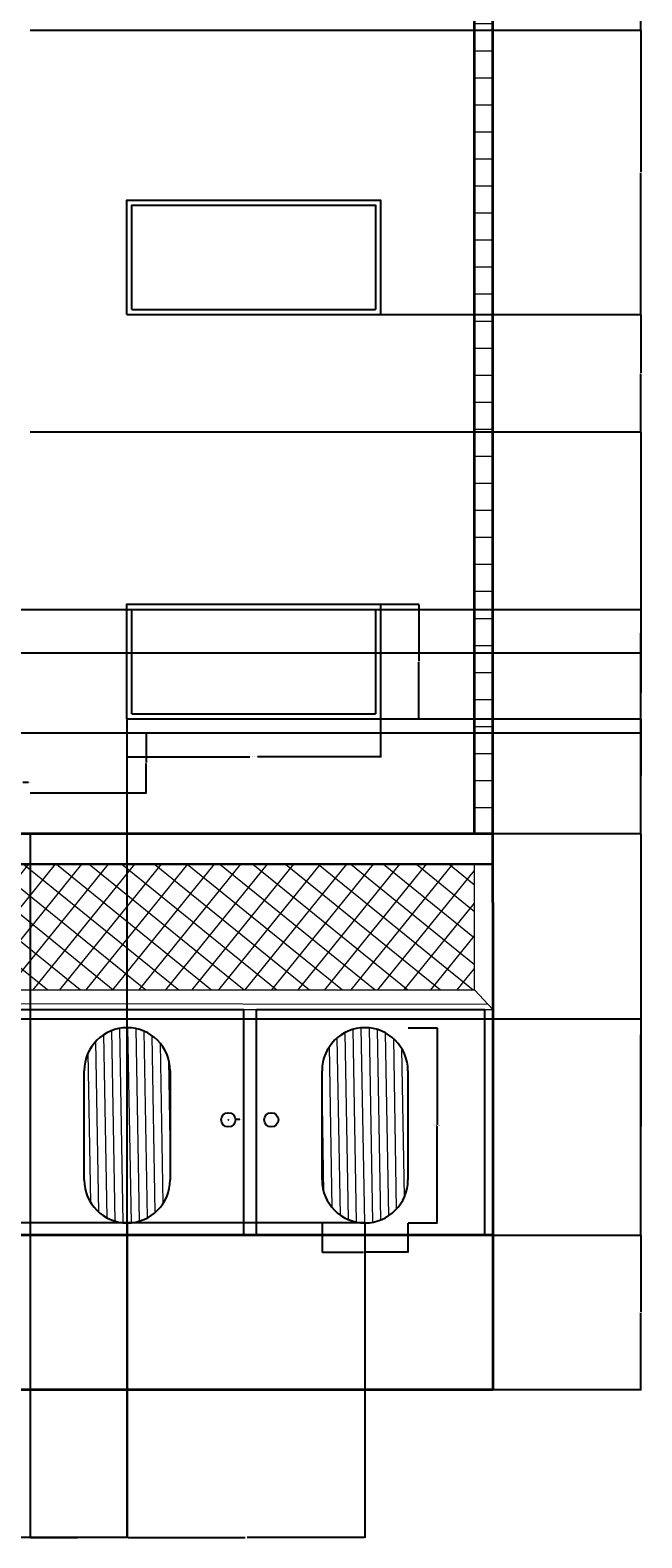
# Model space of a CAD drawing. Units: inches. Extents: x 373 to 969, y 157 to 1341.
# Tile 2 of 3: x 731 to 969, y 157 to 743. Entities that reach past the tile are written whole.
import ezdxf

# ---------------------------------------------------------------- set-up
doc = ezdxf.new("R2010")
doc.units = ezdxf.units.IN
doc.header["$MEASUREMENT"] = 0
for name, color, linetype, lineweight in [('A-ANNO-DIMS', 2, 'Continuous', 18), ('A-DOOR', 3, 'Continuous', 25), ('A-DOOR-PATT', 8, 'Continuous', 13), ('A-ELEV-TRIM', 9, 'Continuous', 18), ('A-FLOR', 7, 'Continuous', 30), ('A-GLAZ', 4, 'Continuous', 25), ('A-WALL', 7, 'Continuous', 35), ('A-WALL-PATT', 8, 'Continuous', 13)]:
    doc.layers.add(name, color=color, linetype=linetype, lineweight=lineweight)
doc.styles.get("Standard").update_dxf_attribs({"font": 'arial.ttf'})
doc.dimstyles.get("Standard").update_dxf_attribs({"dimtxt": 0.18, "dimasz": 0.18, "dimexe": 0.18, "dimexo": 0.0625, "dimgap": 0.09, "dimtad": 0, "dimtih": 1, "dimtoh": 1, "dimdec": 4, "dimzin": 0, "dimdsep": 46, "dimlunit": 4, "dimtxsty": 'Standard', "dimcen": 0.09, "dimadec": 0, "dimazin": 0, "dimtfac": 1, "dimtdec": 4, "dimtofl": 0, "dimtmove": 0, "dimatfit": 3, "dimfxl": 1, "dimtolj": 1, "dimtzin": 0, "dimarcsym": 0})

# ---------------------------------------------------------------- blocks, each defined once
blk = doc.blocks.new('WIN-FIXED-FRAME-ELEV')
for p, q in [((0, 0), (98.59, 0)), ((2, 2), (96.59, 2))]:
    blk.add_line(p, q)
for points in [[(0, 0), (0, 44.5), (98.59, 44.5), (98.59, 0)], [(2, 2), (2, 42.5), (96.59, 42.5), (96.59, 2)]]:
    blk.add_lwpolyline(points)
blk = doc.blocks.new('DOOR-OBROUND-INSERT-ELEV')
for points in [[(0, 16.68), (0, 59.13)], [(33.36, 59.13), (33.36, 16.68)]]:
    blk.add_lwpolyline(points)
for centre, start, end in [((16.68, 59.13), 0, 180), ((16.68, 16.68), 180, 0)]:
    blk.add_arc(centre, 16.68, start, end)
blk = doc.blocks.new('*D7')
at = {"layer": 'A-ANNO-DIMS', "color": 0, "lineweight": -2, "transparency": 16777216}
for p, q in [((768.48, 475.42), (768.48, 460.52)), ((867.07, 475.42), (867.07, 460.52)), ((768.66, 460.7), (816.26, 460.7)), ((866.89, 460.7), (819.29, 460.7))]:
    blk.add_line(p, q, dxfattribs=at)
at = {"layer": 'A-ANNO-DIMS', "color": 0, "transparency": 16777216}
for points in [[(768.66, 460.73), (768.66, 460.67), (768.48, 460.7)], [(866.89, 460.73), (866.89, 460.67), (867.07, 460.7)]]:
    blk.add_solid(points, dxfattribs=at)
at = {"layer": 'Defpoints', "color": 0, "transparency": 16777216}
for p in [(768.48, 475.48), (867.07, 475.48), (867.07, 460.7)]:
    blk.add_point(p, dxfattribs=at)
at = {"layer": 'A-ANNO-DIMS', "color": 0, "transparency": 16777216, "insert": (817.77, 460.7), "char_height": 0.18, "attachment_point": 5}
blk.add_mtext('\\A1;FIXED WINDOW 99 TYP.', dxfattribs=at)
blk = doc.blocks.new('*D8')
at = {"layer": 'A-ANNO-DIMS', "color": 0, "lineweight": -2, "transparency": 16777216}
for p, q in [((867.13, 519.98), (882.04, 519.98)), ((881.86, 519.8), (881.86, 497.92)), ((881.86, 475.66), (881.86, 497.55)), ((867.13, 475.48), (882.04, 475.48))]:
    blk.add_line(p, q, dxfattribs=at)
at = {"layer": 'A-ANNO-DIMS', "color": 0, "transparency": 16777216}
for points in [[(881.83, 519.8), (881.89, 519.8), (881.86, 519.98)], [(881.83, 475.66), (881.89, 475.66), (881.86, 475.48)]]:
    blk.add_solid(points, dxfattribs=at)
at = {"layer": 'Defpoints', "color": 0, "transparency": 16777216}
for p in [(867.07, 519.98), (881.86, 519.98), (867.07, 475.48)]:
    blk.add_point(p, dxfattribs=at)
at = {"layer": 'A-ANNO-DIMS', "color": 0, "transparency": 16777216, "insert": (881.86, 497.73), "char_height": 0.18, "attachment_point": 5}
blk.add_mtext('\\A1;45 TYP.', dxfattribs=at)
blk = doc.blocks.new('*D12')
at = {"layer": 'A-ANNO-DIMS', "color": 0, "lineweight": -2, "transparency": 16777216}
for p, q in [((731, 469.98), (776.15, 469.98)), ((775.97, 469.8), (775.97, 458.53)), ((775.97, 446.9), (775.97, 458.17)), ((731, 446.72), (776.15, 446.72))]:
    blk.add_line(p, q, dxfattribs=at)
at = {"layer": 'A-ANNO-DIMS', "color": 0, "transparency": 16777216}
for points in [[(775.94, 469.8), (776, 469.8), (775.97, 469.98)], [(775.94, 446.9), (776, 446.9), (775.97, 446.72)]]:
    blk.add_solid(points, dxfattribs=at)
at = {"layer": 'Defpoints', "color": 0, "transparency": 16777216}
for p in [(730.93, 469.98), (775.97, 469.98), (730.93, 446.72)]:
    blk.add_point(p, dxfattribs=at)
at = {"layer": 'A-ANNO-DIMS', "color": 0, "transparency": 16777216, "insert": (775.97, 458.35), "char_height": 0.18, "attachment_point": 5}
blk.add_mtext('\\A1;23 TYP.', dxfattribs=at)
blk = doc.blocks.new('*D13')
at = {"layer": 'A-ANNO-DIMS', "color": 0, "lineweight": -2, "transparency": 16777216}
for p, q in [((877.72, 355.49), (889.2, 355.49)), ((889.02, 355.31), (889.02, 317.77)), ((889.02, 279.87), (889.02, 317.41)), ((877.72, 279.69), (889.2, 279.69))]:
    blk.add_line(p, q, dxfattribs=at)
at = {"layer": 'A-ANNO-DIMS', "color": 0, "transparency": 16777216}
for points in [[(888.99, 355.31), (889.05, 355.31), (889.02, 355.49)], [(888.99, 279.87), (889.05, 279.87), (889.02, 279.69)]]:
    blk.add_solid(points, dxfattribs=at)
at = {"layer": 'Defpoints', "color": 0, "transparency": 16777216}
for p in [(877.65, 355.49), (889.02, 355.49), (877.65, 279.69)]:
    blk.add_point(p, dxfattribs=at)
at = {"layer": 'A-ANNO-DIMS', "color": 0, "transparency": 16777216, "insert": (889.02, 317.59), "char_height": 0.18, "attachment_point": 5}
blk.add_mtext('\\A1;DOOR INSERT 76 TYP.', dxfattribs=at)
blk = doc.blocks.new('*D14')
at = {"layer": 'A-ANNO-DIMS', "color": 0, "lineweight": -2, "transparency": 16777216}
for p, q in [((844.3, 279.62), (844.3, 268.14)), ((877.65, 279.62), (877.65, 268.14)), ((844.48, 268.32), (860.45, 268.32)), ((877.47, 268.32), (861.5, 268.32))]:
    blk.add_line(p, q, dxfattribs=at)
at = {"layer": 'A-ANNO-DIMS', "color": 0, "transparency": 16777216}
for points in [[(844.48, 268.35), (844.48, 268.29), (844.3, 268.32)], [(877.47, 268.35), (877.47, 268.29), (877.65, 268.32)]]:
    blk.add_solid(points, dxfattribs=at)
at = {"layer": 'Defpoints', "color": 0, "transparency": 16777216}
for p in [(844.3, 279.69), (877.65, 279.69), (877.65, 268.32)]:
    blk.add_point(p, dxfattribs=at)
at = {"layer": 'A-ANNO-DIMS', "color": 0, "transparency": 16777216, "insert": (860.97, 268.32), "char_height": 0.18, "attachment_point": 5}
blk.add_mtext('\\A1;33 TYP.', dxfattribs=at)
blk = doc.blocks.new('*D15')
at = {"layer": 'A-ANNO-DIMS', "color": 0, "lineweight": -2, "transparency": 16777216}
for p, q in [((910.76, 274.98), (968.33, 274.98)), ((968.15, 274.8), (968.15, 245.17)), ((968.15, 215.16), (968.15, 244.8)), ((910.76, 214.98), (968.33, 214.98))]:
    blk.add_line(p, q, dxfattribs=at)
at = {"layer": 'A-ANNO-DIMS', "color": 0, "transparency": 16777216}
for points in [[(968.12, 274.8), (968.18, 274.8), (968.15, 274.98)], [(968.12, 215.16), (968.18, 215.16), (968.15, 214.98)]]:
    blk.add_solid(points, dxfattribs=at)
at = {"layer": 'Defpoints', "color": 0, "transparency": 16777216}
for p in [(910.7, 274.98), (968.15, 274.98), (910.7, 214.98)]:
    blk.add_point(p, dxfattribs=at)
at = {"layer": 'A-ANNO-DIMS', "color": 0, "transparency": 16777216, "insert": (968.15, 244.98), "char_height": 0.18, "attachment_point": 5}
blk.add_mtext('\\A1;60', dxfattribs=at)
blk = doc.blocks.new('*D16')
at = {"layer": 'A-ANNO-DIMS', "color": 0, "lineweight": -2, "transparency": 16777216}
for p, q in [((910.76, 430.98), (968.33, 430.98)), ((968.15, 430.8), (968.15, 353.17)), ((968.15, 275.16), (968.15, 352.8)), ((910.76, 274.98), (968.33, 274.98))]:
    blk.add_line(p, q, dxfattribs=at)
at = {"layer": 'A-ANNO-DIMS', "color": 0, "transparency": 16777216}
for points in [[(968.12, 430.8), (968.18, 430.8), (968.15, 430.98)], [(968.12, 275.16), (968.18, 275.16), (968.15, 274.98)]]:
    blk.add_solid(points, dxfattribs=at)
at = {"layer": 'Defpoints', "color": 0, "transparency": 16777216}
for p in [(910.7, 430.98), (968.15, 430.98), (910.7, 274.98)]:
    blk.add_point(p, dxfattribs=at)
at = {"layer": 'A-ANNO-DIMS', "color": 0, "transparency": 16777216, "insert": (968.15, 352.98), "char_height": 0.18, "attachment_point": 5}
blk.add_mtext('\\A1;156', dxfattribs=at)
blk = doc.blocks.new('*D17')
at = {"layer": 'A-ANNO-DIMS', "color": 0, "lineweight": -2, "transparency": 16777216}
for p, q in [((731, 586.98), (968.33, 586.98)), ((968.15, 586.8), (968.15, 509.17)), ((968.15, 431.16), (968.15, 508.8)), ((910.76, 430.98), (968.33, 430.98))]:
    blk.add_line(p, q, dxfattribs=at)
at = {"layer": 'A-ANNO-DIMS', "color": 0, "transparency": 16777216}
for points in [[(968.12, 586.8), (968.18, 586.8), (968.15, 586.98)], [(968.12, 431.16), (968.18, 431.16), (968.15, 430.98)]]:
    blk.add_solid(points, dxfattribs=at)
at = {"layer": 'Defpoints', "color": 0, "transparency": 16777216}
for p in [(730.93, 586.98), (968.15, 586.98), (910.7, 430.98)]:
    blk.add_point(p, dxfattribs=at)
at = {"layer": 'A-ANNO-DIMS', "color": 0, "transparency": 16777216, "insert": (968.15, 508.98), "char_height": 0.18, "attachment_point": 5}
blk.add_mtext('\\A1;156', dxfattribs=at)
blk = doc.blocks.new('*D18')
at = {"layer": 'A-ANNO-DIMS', "color": 0, "lineweight": -2, "transparency": 16777216}
for p, q in [((867.13, 632.48), (968.33, 632.48)), ((968.15, 632.3), (968.15, 609.92)), ((968.15, 587.16), (968.15, 609.55)), ((731, 586.98), (968.33, 586.98))]:
    blk.add_line(p, q, dxfattribs=at)
at = {"layer": 'A-ANNO-DIMS', "color": 0, "transparency": 16777216}
for points in [[(968.12, 632.3), (968.18, 632.3), (968.15, 632.48)], [(968.12, 587.16), (968.18, 587.16), (968.15, 586.98)]]:
    blk.add_solid(points, dxfattribs=at)
at = {"layer": 'Defpoints', "color": 0, "transparency": 16777216}
for p in [(867.07, 632.48), (968.15, 632.48), (730.93, 586.98)]:
    blk.add_point(p, dxfattribs=at)
at = {"layer": 'A-ANNO-DIMS', "color": 0, "transparency": 16777216, "insert": (968.15, 609.73), "char_height": 0.18, "attachment_point": 5}
blk.add_mtext('\\A1;45.5', dxfattribs=at)
blk = doc.blocks.new('*D19')
at = {"layer": 'A-ANNO-DIMS', "color": 0, "lineweight": -2, "transparency": 16777216}
for p, q in [((731, 742.98), (968.33, 742.98)), ((968.15, 742.8), (968.15, 687.92)), ((968.15, 632.66), (968.15, 687.55)), ((867.13, 632.48), (968.33, 632.48))]:
    blk.add_line(p, q, dxfattribs=at)
at = {"layer": 'A-ANNO-DIMS', "color": 0, "transparency": 16777216}
for points in [[(968.12, 742.8), (968.18, 742.8), (968.15, 742.98)], [(968.12, 632.66), (968.18, 632.66), (968.15, 632.48)]]:
    blk.add_solid(points, dxfattribs=at)
at = {"layer": 'Defpoints', "color": 0, "transparency": 16777216}
for p in [(730.93, 742.98), (968.15, 742.98), (867.07, 632.48)]:
    blk.add_point(p, dxfattribs=at)
at = {"layer": 'A-ANNO-DIMS', "color": 0, "transparency": 16777216, "insert": (968.15, 687.73), "char_height": 0.18, "attachment_point": 5}
blk.add_mtext('\\A1;110.5', dxfattribs=at)
blk = doc.blocks.new('*D20')
at = {"layer": 'A-ANNO-DIMS', "color": 0, "lineweight": -2, "transparency": 16777216}
for p, q in [((867.13, 789.48), (968.33, 789.48)), ((968.15, 789.3), (968.15, 766.42)), ((968.15, 743.16), (968.15, 766.05)), ((731, 742.98), (968.33, 742.98))]:
    blk.add_line(p, q, dxfattribs=at)
at = {"layer": 'A-ANNO-DIMS', "color": 0, "transparency": 16777216}
for points in [[(968.12, 789.3), (968.18, 789.3), (968.15, 789.48)], [(968.12, 743.16), (968.18, 743.16), (968.15, 742.98)]]:
    blk.add_solid(points, dxfattribs=at)
at = {"layer": 'Defpoints', "color": 0, "transparency": 16777216}
for p in [(867.07, 789.48), (968.15, 789.48), (730.93, 742.98)]:
    blk.add_point(p, dxfattribs=at)
at = {"layer": 'A-ANNO-DIMS', "color": 0, "transparency": 16777216, "insert": (968.15, 766.23), "char_height": 0.18, "attachment_point": 5}
blk.add_mtext('\\A1;46.5', dxfattribs=at)
blk = doc.blocks.new('*D25')
at = {"layer": 'A-ANNO-DIMS', "color": 0, "lineweight": -2, "transparency": 16777216}
for p, q in [((768.48, 475.42), (768.48, 157.35)), ((730.93, 430.92), (730.93, 157.35)), ((731.11, 157.53), (749.31, 157.53)), ((768.3, 157.53), (750.1, 157.53))]:
    blk.add_line(p, q, dxfattribs=at)
at = {"layer": 'A-ANNO-DIMS', "color": 0, "transparency": 16777216}
for points in [[(731.11, 157.56), (731.11, 157.5), (730.93, 157.53)], [(768.3, 157.56), (768.3, 157.5), (768.48, 157.53)]]:
    blk.add_solid(points, dxfattribs=at)
at = {"layer": 'Defpoints', "color": 0, "transparency": 16777216}
for p in [(768.48, 475.48), (730.93, 430.98), (768.48, 157.53)]:
    blk.add_point(p, dxfattribs=at)
at = {"layer": 'A-ANNO-DIMS', "color": 0, "transparency": 16777216, "insert": (749.7, 157.53), "char_height": 0.18, "attachment_point": 5}
blk.add_mtext('\\A1;37.54', dxfattribs=at)
blk = doc.blocks.new('*D26')
at = {"layer": 'A-ANNO-DIMS', "color": 0, "lineweight": -2, "transparency": 16777216}
for p, q in [((867.13, 475.48), (968.33, 475.48)), ((968.15, 475.3), (968.15, 453.42)), ((968.15, 431.16), (968.15, 453.05)), ((910.76, 430.98), (968.33, 430.98))]:
    blk.add_line(p, q, dxfattribs=at)
at = {"layer": 'A-ANNO-DIMS', "color": 0, "transparency": 16777216}
for points in [[(968.12, 475.3), (968.18, 475.3), (968.15, 475.48)], [(968.12, 431.16), (968.18, 431.16), (968.15, 430.98)]]:
    blk.add_solid(points, dxfattribs=at)
at = {"layer": 'Defpoints', "color": 0, "transparency": 16777216}
for p in [(867.07, 475.48), (910.7, 430.98), (968.15, 430.98)]:
    blk.add_point(p, dxfattribs=at)
at = {"layer": 'A-ANNO-DIMS', "color": 0, "transparency": 16777216, "insert": (968.15, 453.23), "char_height": 0.18, "attachment_point": 5}
blk.add_mtext('\\A1;44.5', dxfattribs=at)
blk = doc.blocks.new('*D30')
at = {"layer": 'A-ANNO-DIMS', "color": 0, "lineweight": -2, "transparency": 16777216}
for p, q in [((490.76, 517.98), (968.33, 517.98)), ((968.15, 517.8), (968.15, 494.17)), ((968.15, 470.16), (968.15, 493.8)), ((490.76, 469.98), (968.33, 469.98))]:
    blk.add_line(p, q, dxfattribs=at)
at = {"layer": 'A-ANNO-DIMS', "color": 0, "transparency": 16777216}
for points in [[(968.12, 517.8), (968.18, 517.8), (968.15, 517.98)], [(968.12, 470.16), (968.18, 470.16), (968.15, 469.98)]]:
    blk.add_solid(points, dxfattribs=at)
at = {"layer": 'Defpoints', "color": 0, "transparency": 16777216}
for p in [(490.7, 517.98), (968.15, 517.98), (490.7, 469.98)]:
    blk.add_point(p, dxfattribs=at)
at = {"layer": 'A-ANNO-DIMS', "color": 0, "transparency": 16777216, "insert": (968.15, 493.98), "char_height": 0.18, "attachment_point": 5}
blk.add_mtext('\\A1;48', dxfattribs=at)
blk = doc.blocks.new('*D35')
at = {"layer": 'A-ANNO-DIMS', "color": 0, "lineweight": -2, "transparency": 16777216}
for p, q in [((520.86, 358.98), (968.33, 358.98)), ((968.15, 358.8), (968.15, 317.17)), ((968.15, 275.16), (968.15, 316.8)), ((520.86, 274.98), (968.33, 274.98))]:
    blk.add_line(p, q, dxfattribs=at)
at = {"layer": 'A-ANNO-DIMS', "color": 0, "transparency": 16777216}
for points in [[(968.12, 358.8), (968.18, 358.8), (968.15, 358.98)], [(968.12, 275.16), (968.18, 275.16), (968.15, 274.98)]]:
    blk.add_solid(points, dxfattribs=at)
at = {"layer": 'Defpoints', "color": 0, "transparency": 16777216}
for p in [(520.8, 358.98), (968.15, 358.98), (520.8, 274.98)]:
    blk.add_point(p, dxfattribs=at)
at = {"layer": 'A-ANNO-DIMS', "color": 0, "transparency": 16777216, "insert": (968.15, 316.98), "char_height": 0.18, "attachment_point": 5}
blk.add_mtext('\\A1;84', dxfattribs=at)
blk = doc.blocks.new('*D40')
at = {"layer": 'A-ANNO-DIMS', "color": 0, "lineweight": -2, "transparency": 16777216}
for p, q in [((675.1, 279.62), (675.1, 157.35)), ((768.63, 279.62), (768.63, 157.35)), ((675.28, 157.53), (721.47, 157.53)), ((768.45, 157.53), (722.26, 157.53))]:
    blk.add_line(p, q, dxfattribs=at)
at = {"layer": 'A-ANNO-DIMS', "color": 0, "transparency": 16777216}
for points in [[(675.28, 157.56), (675.28, 157.5), (675.1, 157.53)], [(768.45, 157.56), (768.45, 157.5), (768.63, 157.53)]]:
    blk.add_solid(points, dxfattribs=at)
at = {"layer": 'Defpoints', "color": 0, "transparency": 16777216}
for p in [(675.1, 279.69), (768.63, 279.69), (768.63, 157.53)]:
    blk.add_point(p, dxfattribs=at)
at = {"layer": 'A-ANNO-DIMS', "color": 0, "transparency": 16777216, "insert": (721.86, 157.53), "char_height": 0.18, "attachment_point": 5}
blk.add_mtext('\\A1;93.53', dxfattribs=at)
blk = doc.blocks.new('*D41')
at = {"layer": 'A-ANNO-DIMS', "color": 0, "lineweight": -2, "transparency": 16777216}
for p, q in [((768.63, 279.62), (768.63, 157.35)), ((860.97, 279.62), (860.97, 157.35)), ((768.81, 157.53), (814.41, 157.53)), ((860.79, 157.53), (815.2, 157.53))]:
    blk.add_line(p, q, dxfattribs=at)
at = {"layer": 'A-ANNO-DIMS', "color": 0, "transparency": 16777216}
for points in [[(768.81, 157.56), (768.81, 157.5), (768.63, 157.53)], [(860.79, 157.56), (860.79, 157.5), (860.97, 157.53)]]:
    blk.add_solid(points, dxfattribs=at)
at = {"layer": 'Defpoints', "color": 0, "transparency": 16777216}
for p in [(768.63, 279.69), (860.97, 279.69), (860.97, 157.53)]:
    blk.add_point(p, dxfattribs=at)
at = {"layer": 'A-ANNO-DIMS', "color": 0, "transparency": 16777216, "insert": (814.8, 157.53), "char_height": 0.18, "attachment_point": 5}
blk.add_mtext('\\A1;92.35', dxfattribs=at)
blk = doc.blocks.new('*D44')
at = {"layer": 'A-ANNO-DIMS', "color": 0, "lineweight": -2, "transparency": 16777216}
for p, q in [((860.91, 279.69), (373.07, 279.69)), ((373.25, 279.51), (373.25, 277.52)), ((373.25, 275.16), (373.25, 277.15)), ((818.75, 274.98), (373.07, 274.98))]:
    blk.add_line(p, q, dxfattribs=at)
at = {"layer": 'A-ANNO-DIMS', "color": 0, "transparency": 16777216}
for points in [[(373.22, 279.51), (373.28, 279.51), (373.25, 279.69)], [(373.22, 275.16), (373.28, 275.16), (373.25, 274.98)]]:
    blk.add_solid(points, dxfattribs=at)
at = {"layer": 'Defpoints', "color": 0, "transparency": 16777216}
for p in [(373.25, 279.69), (860.97, 279.69), (818.82, 274.98)]:
    blk.add_point(p, dxfattribs=at)
at = {"layer": 'A-ANNO-DIMS', "color": 0, "transparency": 16777216, "insert": (373.25, 277.34), "char_height": 0.18, "attachment_point": 5}
blk.add_mtext('\\A1;4.702', dxfattribs=at)
blk = doc.blocks.new('*D45')
at = {"layer": 'A-ANNO-DIMS', "color": 0, "lineweight": -2, "transparency": 16777216}
for p, q in [((709.67, 501.13), (968.33, 501.13)), ((968.15, 500.95), (968.15, 485.74)), ((968.15, 470.16), (968.15, 485.38)), ((721.89, 469.98), (968.33, 469.98))]:
    blk.add_line(p, q, dxfattribs=at)
at = {"layer": 'A-ANNO-DIMS', "color": 0, "transparency": 16777216}
for points in [[(968.12, 500.95), (968.18, 500.95), (968.15, 501.13)], [(968.12, 470.16), (968.18, 470.16), (968.15, 469.98)]]:
    blk.add_solid(points, dxfattribs=at)
at = {"layer": 'Defpoints', "color": 0, "transparency": 16777216}
for p in [(709.61, 501.13), (968.15, 501.13), (721.82, 469.98)]:
    blk.add_point(p, dxfattribs=at)
at = {"layer": 'A-ANNO-DIMS', "color": 0, "transparency": 16777216, "insert": (968.15, 485.56), "char_height": 0.18, "attachment_point": 5}
blk.add_mtext('\\A1;31.146', dxfattribs=at)
blk = doc.blocks.new('*D55')
at = {"layer": 'A-ANNO-DIMS', "color": 0, "lineweight": -2, "transparency": 16777216}
for p, q in [((734.58, 1283.61), (373.07, 1283.61)), ((373.25, 1283.43), (373.25, 749.48)), ((373.25, 215.16), (373.25, 749.11)), ((430.64, 214.98), (373.07, 214.98))]:
    blk.add_line(p, q, dxfattribs=at)
at = {"layer": 'A-ANNO-DIMS', "color": 0, "transparency": 16777216}
for points in [[(373.22, 1283.43), (373.28, 1283.43), (373.25, 1283.61)], [(373.22, 215.16), (373.28, 215.16), (373.25, 214.98)]]:
    blk.add_solid(points, dxfattribs=at)
at = {"layer": 'Defpoints', "color": 0, "transparency": 16777216}
for p in [(373.25, 1283.61), (734.64, 1283.61), (430.7, 214.98)]:
    blk.add_point(p, dxfattribs=at)
at = {"layer": 'A-ANNO-DIMS', "color": 0, "transparency": 16777216, "insert": (373.25, 749.3), "char_height": 0.18, "attachment_point": 5}
blk.add_mtext('\\A1;1068.6', dxfattribs=at)
blk = doc.blocks.new('*D58')
at = {"layer": 'A-ANNO-DIMS', "color": 0, "lineweight": -2, "transparency": 16777216}
for p, q in [((723.88, 450.69), (724.06, 450.69)), ((723.97, 450.6), (723.97, 450.78)), ((730.33, 450.7), (728.12, 450.7))]:
    blk.add_line(p, q, dxfattribs=at)
at = {"layer": 'A-ANNO-DIMS', "color": 0, "transparency": 16777216}
blk.add_solid([(728.12, 450.73), (728.12, 450.67), (727.94, 450.7)], dxfattribs=at)
at = {"layer": 'Defpoints', "color": 0, "transparency": 16777216}
for p in [(720, 450.69), (727.94, 450.7)]:
    blk.add_point(p, dxfattribs=at)
at = {"layer": 'A-ANNO-DIMS', "color": 0, "transparency": 16777216, "insert": (731.01, 450.7), "char_height": 0.18, "attachment_point": 5}
blk.add_mtext('\\A1;4X ∅7.946', dxfattribs=at)
blk = doc.blocks.new('*D60')
at = {"layer": 'A-ANNO-DIMS', "color": 0, "lineweight": -2, "transparency": 16777216}
for p, q in [((807.82, 319.72), (808, 319.72)), ((807.91, 319.63), (807.91, 319.81)), ((812.35, 319.85), (810.86, 319.8))]:
    blk.add_line(p, q, dxfattribs=at)
at = {"layer": 'A-ANNO-DIMS', "color": 0, "transparency": 16777216}
blk.add_solid([(810.86, 319.83), (810.87, 319.77), (810.68, 319.8)], dxfattribs=at)
at = {"layer": 'Defpoints', "color": 0, "transparency": 16777216}
for p in [(805.13, 319.64), (810.68, 319.8)]:
    blk.add_point(p, dxfattribs=at)
at = {"layer": 'A-ANNO-DIMS', "color": 0, "transparency": 16777216, "insert": (813.03, 319.85), "char_height": 0.18, "attachment_point": 5}
blk.add_mtext('\\A1;3X ∅5.553', dxfattribs=at)

msp = doc.modelspace()

# ---------------------------------------------------------------- hatches: boundary and pattern name
at = {"layer": 'A-DOOR-PATT'}
h = msp.add_hatch(dxfattribs=at)
h.set_pattern_fill('ANSI31', color=256, scale=25, angle=226)
h.paths.add_polyline_path([(785.3076, 338.8165, 1), (751.9521, 338.8165), (751.9521, 296.364, 1), (785.3076, 296.364)])
h.paths.add_polyline_path([(877.6527, 338.8165, 1), (844.2972, 338.8165), (844.2972, 296.364, 1), (877.6527, 296.364)])
at = {"layer": 'A-WALL-PATT'}
h = msp.add_hatch(dxfattribs=at)
h.set_pattern_fill('ANSI31', color=256, scale=84, angle=315)
h.paths.add_polyline_path([(910.6998, 1276.1757), (903.5487, 1276.1757), (903.5487, 430.9843), (910.6998, 430.9843)])
h = msp.add_hatch(dxfattribs=at)
h.set_pattern_fill('ANSI37', color=256, scale=64, angle=96)
h.paths.add_polyline_path([(903.5487, 418.9843), (632.3184, 418.9843), (632.3184, 370.2071), (903.5487, 370.2071)])

# ---------------------------------------------------------------- linework, layer by layer
at = {"layer": 'A-DOOR'}
for points in [[(725.2573, 362.6044), (813.8375, 362.6044), (813.8375, 274.9843), (725.2573, 274.9843)], [(818.8151, 362.6044), (907.3953, 362.6044), (907.3953, 274.9843), (818.8151, 274.9843)]]:
    msp.add_lwpolyline(points, close=True, dxfattribs=at)
for centre in [(807.9093, 319.7202), (824.5813, 319.7202)]:
    msp.add_circle(centre, 2.7765, dxfattribs=at)
at = {"layer": 'A-ELEV-TRIM'}
for p, q in [((903.5487, 370.2071), (903.5487, 418.9843)), ((632.3184, 370.2071), (903.5487, 370.2071)), ((910.6998, 362.6044), (903.5487, 370.2071)), ((624.5243, 364.9818), (908.76, 364.6667)), ((620.9782, 362.6044), (910.6998, 362.6044))]:
    msp.add_line(p, q, dxfattribs=at)
at = {"layer": 'A-FLOR'}
msp.add_line((430.6998, 418.9843), (910.6998, 418.9843), dxfattribs=at)
at = {"layer": 'A-WALL'}
for p, q in [((903.5487, 430.9843), (903.5487, 1283.6064)), ((910.6998, 404.1026), (910.6998, 430.9843)), ((910.6998, 404.1026), (910.6998, 214.9843)), ((910.6998, 274.9843), (430.6998, 274.9843)), ((430.6998, 214.9843), (910.6998, 214.9843))]:
    msp.add_line(p, q, dxfattribs=at)
msp.add_lwpolyline([(430.6998, 430.9843), (910.6998, 430.9843), (910.6998, 1276.1757)], dxfattribs=at)

# ---------------------------------------------------------------- block references
at = {"layer": 'A-DOOR'}
for p in [(751.952, 279.686), (844.2971, 279.686)]:
    msp.add_blockref('DOOR-OBROUND-INSERT-ELEV', p, dxfattribs=at)
at = {"layer": 'A-GLAZ'}
for p in [(768.476, 632.484), (768.476, 475.484)]:
    msp.add_blockref('WIN-FIXED-FRAME-ELEV', p, dxfattribs=at)

# ---------------------------------------------------------------- dimensions: what is measured, and where the dimension line sits
at = {"layer": 'A-ANNO-DIMS'}
for base, p1, p2, override, picture, middle in [((373.2498, 1283.6064), (430.6998, 214.9843), (734.6424, 1283.6064), {"dimdec": 1, "dimlfac": 1, "dimrnd": 0, "dimzin": 0, "dimdsep": 46, "dimlunit": 2}, '*D55', (373.2498, 749.2954)), ((968.1498, 789.4843), (730.9335, 742.9843), (867.0679, 789.4843), {"dimdec": 1, "dimlfac": 1, "dimrnd": 0, "dimzin": 0, "dimdsep": 46, "dimlunit": 2}, '*D20', (968.1498, 766.2343)), ((968.1498, 742.9843), (867.0679, 632.4843), (730.9335, 742.9843), {"dimdec": 1, "dimlfac": 1, "dimrnd": 0, "dimzin": 0, "dimdsep": 46, "dimlunit": 2}, '*D19', (968.1498, 687.7343)), ((968.1498, 632.4843), (730.9335, 586.9843), (867.0679, 632.4843), {"dimdec": 1, "dimlfac": 1, "dimrnd": 0, "dimzin": 0, "dimdsep": 46, "dimlunit": 2}, '*D18', (968.1498, 609.7343)), ((968.1498, 586.9843), (910.6998, 430.9843), (730.9335, 586.9843), {"dimdec": 0, "dimlfac": 1, "dimrnd": 0, "dimzin": 0, "dimdsep": 46, "dimlunit": 2}, '*D17', (968.1498, 508.9843)), ((968.1498, 517.9843), (490.6998, 469.9843), (490.6998, 517.9843), {"dimdec": 0, "dimlfac": 1, "dimrnd": 0, "dimzin": 0, "dimdsep": 46, "dimlunit": 2}, '*D30', (968.1498, 493.9843)), ((968.1498, 501.1302), (721.8241, 469.9843), (709.6057, 501.1302), {"dimdec": 3, "dimlfac": 1, "dimrnd": 0, "dimzin": 0, "dimdsep": 46, "dimlunit": 2}, '*D45', (968.1498, 485.5573)), ((968.1498, 430.9843), (867.0679, 475.4843), (910.6998, 430.9843), {"dimdec": 1, "dimlfac": 1, "dimrnd": 0, "dimzin": 0, "dimdsep": 46, "dimlunit": 2}, '*D26', (968.1498, 453.2343)), ((968.1498, 430.9843), (910.6998, 274.9843), (910.6998, 430.9843), {"dimdec": 0, "dimlfac": 1, "dimrnd": 0, "dimzin": 0, "dimdsep": 46, "dimlunit": 2}, '*D16', (968.1498, 352.9843)), ((968.1498, 358.9843), (520.8024, 274.9843), (520.8024, 358.9843), {"dimdec": 0, "dimlfac": 1, "dimrnd": 0, "dimzin": 0, "dimdsep": 46, "dimlunit": 2}, '*D35', (968.1498, 316.9843)), ((373.2498, 279.6862), (818.8151, 274.9843), (860.9749, 279.6862), {"dimdec": 3, "dimlfac": 1, "dimrnd": 0, "dimzin": 0, "dimdsep": 46, "dimlunit": 2}, '*D44', (373.2498, 277.3353)), ((968.1498, 274.9843), (910.6998, 214.9843), (910.6998, 274.9843), {"dimdec": 0, "dimlfac": 1, "dimrnd": 0, "dimzin": 0, "dimdsep": 46, "dimlunit": 2}, '*D15', (968.1498, 244.9843))]:
    dim = msp.add_linear_dim(base=base, p1=p1, p2=p2, angle=90, dimstyle='Standard', override=override, dxfattribs=at)
    dim.commit()
    dim.dimension.update_dxf_attribs({"geometry": picture, "text_midpoint": middle})
for base, p1, p2, text, picture, middle in [((881.8566081032, 519.9843052359), (867.0678783848, 475.4843052359), (867.0678783848, 519.9843052359), '<> TYP.', '*D8', (881.8566081032, 497.7343052359)), ((775.9685, 469.9843), (730.9335, 446.7217), (730.9335, 469.9843), '<> TYP.', '*D12', (775.9685, 458.353)), ((889.0239, 355.4943), (877.6527, 279.6862), (877.6527, 355.4943), 'DOOR INSERT <> TYP.', '*D13', (889.0239, 317.5903))]:
    dim = msp.add_linear_dim(base=base, p1=p1, p2=p2, angle=90, text=text, dimstyle='Standard', override={"dimdec": 0, "dimlfac": 1, "dimrnd": 0, "dimzin": 0, "dimdsep": 46, "dimlunit": 2}, dxfattribs=at)
    dim.commit()
    dim.dimension.update_dxf_attribs({"geometry": picture, "text_midpoint": middle})
for base, p1, p2, picture, middle in [((768.4763, 157.5343), (730.9335, 430.9843), (768.4763, 475.4843), '*D25', (749.7049, 157.5343)), ((768.6299, 157.5343), (675.0969, 279.6862), (768.6299, 279.6862), '*D40', (721.8634, 157.5343)), ((860.97494, 157.5343), (768.62989, 279.68624), (860.97494, 279.68624), '*D41', (814.80242, 157.5343))]:
    dim = msp.add_linear_dim(base=base, p1=p1, p2=p2, dimstyle='Standard', override={"dimdec": 2, "dimlfac": 1, "dimrnd": 0, "dimzin": 0, "dimdsep": 46, "dimlunit": 2}, dxfattribs=at)
    dim.commit()
    dim.dimension.update_dxf_attribs({"geometry": picture, "text_midpoint": middle})
for base, p1, p2, text, picture, middle in [((867.0679, 460.6956), (768.4763, 475.4843), (867.0679, 475.4843), 'FIXED WINDOW <> TYP.', '*D7', (817.7721, 460.6956)), ((877.6527, 268.315), (844.2972, 279.6862), (877.6527, 279.6862), '<> TYP.', '*D14', (860.9749, 268.315))]:
    dim = msp.add_linear_dim(base=base, p1=p1, p2=p2, text=text, dimstyle='Standard', override={"dimdec": 0, "dimlfac": 1, "dimrnd": 0, "dimzin": 0, "dimdsep": 46, "dimlunit": 2}, dxfattribs=at)
    dim.commit()
    dim.dimension.update_dxf_attribs({"geometry": picture, "text_midpoint": middle})
for p1, p2, text, picture, middle in [((719.9982, 450.6895), (727.9444, 450.7002), '4X <>', '*D58', (730.3283, 450.7034)), ((805.134, 319.6408), (810.6847, 319.7996), '3X <>', '*D60', (812.3499, 319.8472))]:
    dim = msp.add_diameter_dim_2p(p1=p1, p2=p2, text=text, dimstyle='Standard', override={"dimdec": 3, "dimlfac": 1, "dimrnd": 0, "dimzin": 0, "dimdsep": 46, "dimlunit": 2}, dxfattribs=at)
    dim.commit()
    dim.dimension.update_dxf_attribs({"geometry": picture, "text_midpoint": middle, "dimtype": 163})

doc.saveas('drawing.dxf')
